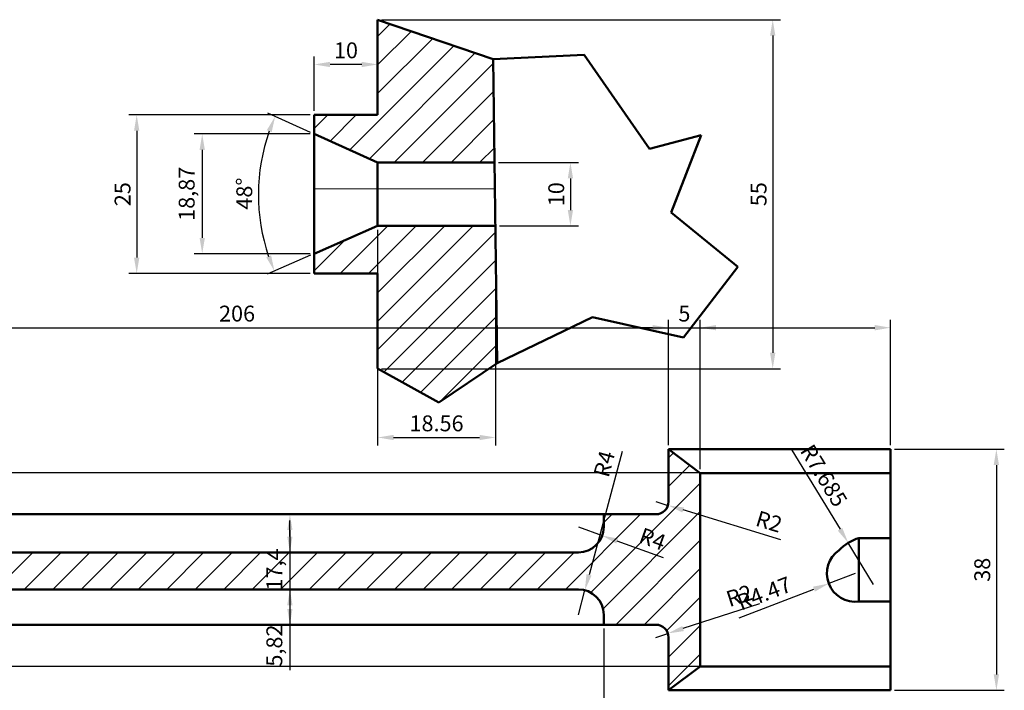
# Model space of a CAD drawing. Units: millimetres. Extents: x 1594 to 1992, y 1694 to 1927.
# Tile 3 of 4: x 1698 to 1853, y 1822 to 1927. Entities that reach past the tile are written whole.
import ezdxf

# ---------------------------------------------------------------- set-up
doc = ezdxf.new("R2010")
doc.units = ezdxf.units.MM
doc.linetypes.add('CENTER', pattern=[50.8, 31.75, -6.35, 6.35, -6.35])
for name, color, linetype, lineweight in [('M-CNTR', 1, 'CENTER', 18), ('M-DIMS', 2, 'Continuous', 25), ('M-HATC', 8, 'Continuous', 18), ('M-OUTL', 7, 'Continuous', 50)]:
    doc.layers.add(name, color=color, linetype=linetype, lineweight=lineweight)
doc.styles.get("Standard").update_dxf_attribs({"font": 'arial.ttf'})
doc.dimstyles.new('ISO-25', dxfattribs={"dimtxt": 2.5, "dimasz": 2.5, "dimexe": 1.25, "dimexo": 0.625, "dimtad": 1, "dimtxsty": 'Standard', "dimcen": 2.5, "dimadec": 0, "dimazin": 0, "dimtfac": 1, "dimtmove": 0, "dimatfit": 3, "dimfxl": 1, "dimarcsym": 0})

# ---------------------------------------------------------------- blocks, each defined once
blk = doc.blocks.new('*D2')
at = {"layer": 'Defpoints', "color": 0, "transparency": 16777216}
for p in [(1834.84, 1859.58), (1834.84, 1821.58), (1851.51, 1821.58)]:
    blk.add_point(p, dxfattribs=at)
at = {"layer": 'M-DIMS', "color": 0, "lineweight": -2, "transparency": 16777216}
for p, q in [((1835.46, 1859.58), (1852.76, 1859.58)), ((1851.51, 1857.08), (1851.51, 1824.08)), ((1835.46, 1821.58), (1852.76, 1821.58))]:
    blk.add_line(p, q, dxfattribs=at)
at = {"layer": 'M-DIMS', "color": 0, "transparency": 16777216}
for points in [[(1851.09, 1857.08), (1851.93, 1857.08), (1851.51, 1859.58)], [(1851.09, 1824.08), (1851.93, 1824.08), (1851.51, 1821.58)]]:
    blk.add_solid(points, dxfattribs=at)
at = {"layer": 'M-DIMS', "color": 0, "transparency": 16777216, "insert": (1849.61, 1840.58), "char_height": 2.5, "attachment_point": 5, "rotation": 90}
blk.add_mtext('38', dxfattribs=at)
blk = doc.blocks.new('*D3')
at = {"layer": 'Defpoints', "color": 0, "transparency": 16777216}
for p in [(1797.84, 1851.32), (1799.75, 1850.73)]:
    blk.add_point(p, dxfattribs=at)
at = {"layer": 'M-DIMS', "color": 0, "lineweight": -2, "transparency": 16777216}
for p, q in [((1797.84, 1851.32), (1799.75, 1850.73)), ((1817.55, 1845.3), (1802.14, 1850))]:
    blk.add_line(p, q, dxfattribs=at)
at = {"layer": 'M-DIMS', "color": 0, "transparency": 16777216}
blk.add_solid([(1802.26, 1850.4), (1802.02, 1849.61), (1799.75, 1850.73)], dxfattribs=at)
at = {"layer": 'M-DIMS', "color": 0, "transparency": 16777216, "insert": (1815.59, 1847.86), "char_height": 2.5, "attachment_point": 5, "rotation": 343.0097}
blk.add_mtext('R2', dxfattribs=at)
blk = doc.blocks.new('*D5')
at = {"layer": 'Defpoints', "color": 0, "transparency": 16777216}
for p in [(1739.34, 1849.32), (1739.34, 1831.92), (1740.17, 1831.92)]:
    blk.add_point(p, dxfattribs=at)
at = {"layer": 'M-DIMS', "color": 0, "lineweight": -2, "transparency": 16777216}
for p, q in [((1739.96, 1849.32), (1741.42, 1849.32)), ((1740.17, 1846.82), (1740.17, 1834.42)), ((1739.96, 1831.92), (1741.42, 1831.92))]:
    blk.add_line(p, q, dxfattribs=at)
at = {"layer": 'M-DIMS', "color": 0, "transparency": 16777216}
for points in [[(1739.75, 1846.82), (1740.58, 1846.82), (1740.17, 1849.32)], [(1739.75, 1834.42), (1740.58, 1834.42), (1740.17, 1831.92)]]:
    blk.add_solid(points, dxfattribs=at)
at = {"layer": 'M-DIMS', "color": 0, "transparency": 16777216, "insert": (1738.04, 1840.62), "char_height": 2.5, "attachment_point": 5, "rotation": 90}
blk.add_mtext('17,4', dxfattribs=at)
blk = doc.blocks.new('*D6')
at = {"layer": 'Defpoints', "color": 0, "transparency": 16777216}
for p in [(1740.17, 1843.32), (1740.17, 1837.49), (1740.17, 1837.49)]:
    blk.add_point(p, dxfattribs=at)
at = {"layer": 'M-DIMS', "color": 0, "lineweight": -2, "transparency": 16777216}
for p, q in [((1740.17, 1845.82), (1740.17, 1848.32)), ((1740.17, 1843.32), (1740.17, 1837.49)), ((1740.79, 1843.32), (1741.42, 1843.32)), ((1740.79, 1837.49), (1741.42, 1837.49)), ((1740.17, 1834.99), (1740.17, 1824.78))]:
    blk.add_line(p, q, dxfattribs=at)
at = {"layer": 'M-DIMS', "color": 0, "transparency": 16777216}
for points in [[(1739.75, 1845.82), (1740.58, 1845.82), (1740.17, 1843.32)], [(1739.75, 1834.99), (1740.58, 1834.99), (1740.17, 1837.49)]]:
    blk.add_solid(points, dxfattribs=at)
at = {"layer": 'M-DIMS', "color": 0, "transparency": 16777216, "insert": (1738.04, 1828.63), "char_height": 2.5, "attachment_point": 5, "rotation": 90}
blk.add_mtext('5,82', dxfattribs=at)
blk = doc.blocks.new('*D7')
at = {"layer": 'Defpoints', "color": 0, "transparency": 16777216}
for p in [(1786.66, 1837.36), (1785.63, 1833.49)]:
    blk.add_point(p, dxfattribs=at)
at = {"layer": 'M-DIMS', "color": 0, "lineweight": -2, "transparency": 16777216}
for p, q in [((1792.51, 1859.24), (1787.31, 1839.77)), ((1785.63, 1833.49), (1786.66, 1837.36))]:
    blk.add_line(p, q, dxfattribs=at)
at = {"layer": 'M-DIMS', "color": 0, "transparency": 16777216}
blk.add_solid([(1786.91, 1839.88), (1787.71, 1839.67), (1786.66, 1837.36)], dxfattribs=at)
at = {"layer": 'M-DIMS', "color": 0, "transparency": 16777216, "insert": (1790.02, 1857.18), "char_height": 2.5, "attachment_point": 5, "rotation": 75.0359}
blk.add_mtext('R4', dxfattribs=at)
blk = doc.blocks.new('*D8')
at = {"layer": 'Defpoints', "color": 0, "transparency": 16777216}
for p in [(1785.63, 1847.32), (1789.39, 1845.96)]:
    blk.add_point(p, dxfattribs=at)
at = {"layer": 'M-DIMS', "color": 0, "lineweight": -2, "transparency": 16777216}
for p, q in [((1785.63, 1847.32), (1789.39, 1845.96)), ((1799.05, 1842.46), (1791.74, 1845.1))]:
    blk.add_line(p, q, dxfattribs=at)
at = {"layer": 'M-DIMS', "color": 0, "transparency": 16777216}
blk.add_solid([(1791.88, 1845.5), (1791.6, 1844.71), (1789.39, 1845.96)], dxfattribs=at)
at = {"layer": 'M-DIMS', "color": 0, "transparency": 16777216, "insert": (1797.21, 1845.12), "char_height": 2.5, "attachment_point": 5, "rotation": 340.0753}
blk.add_mtext('R4', dxfattribs=at)
blk = doc.blocks.new('*D12')
at = {"layer": 'Defpoints', "color": 0, "transparency": 16777216}
for p in [(1797.84, 1829.92), (1799.74, 1830.54)]:
    blk.add_point(p, dxfattribs=at)
at = {"layer": 'M-DIMS', "color": 0, "lineweight": -2, "transparency": 16777216}
for p, q in [((1814.17, 1835.22), (1802.12, 1831.31)), ((1797.84, 1829.92), (1799.74, 1830.54))]:
    blk.add_line(p, q, dxfattribs=at)
at = {"layer": 'M-DIMS', "color": 0, "transparency": 16777216}
blk.add_solid([(1801.99, 1831.71), (1802.25, 1830.91), (1799.74, 1830.54)], dxfattribs=at)
at = {"layer": 'M-DIMS', "color": 0, "transparency": 16777216, "insert": (1811.09, 1836.19), "char_height": 2.5, "attachment_point": 5, "rotation": 17.9685}
blk.add_mtext('R2', dxfattribs=at)
blk = doc.blocks.new('*D34')
at = {"layer": 'Defpoints', "color": 0, "transparency": 16777216}
for p in [(1744, 1909.26), (1754, 1904.77), (1735.52, 1904.02), (1754, 1894.77), (1744, 1890.39)]:
    blk.add_point(p, dxfattribs=at)
at = {"layer": 'M-DIMS', "color": 0, "lineweight": -2, "transparency": 16777216}
for p, q in [((1743.43, 1909.52), (1736.7, 1912.54)), ((1743.43, 1890.14), (1736.59, 1887.15))]:
    blk.add_line(p, q, dxfattribs=at)
blk.add_arc((1765.27, 1899.71), 30.07, 160.5813, 198.8909, dxfattribs=at)
at = {"layer": 'M-DIMS', "color": 0, "transparency": 16777216}
for points in [[(1736.53, 1909.86), (1737.3, 1909.55), (1737.84, 1912.03)], [(1737.21, 1890.13), (1736.44, 1889.83), (1737.73, 1887.65)]]:
    blk.add_solid(points, dxfattribs=at)
at = {"layer": 'M-DIMS', "color": 0, "transparency": 16777216, "insert": (1733.3, 1899.86), "char_height": 2.5, "attachment_point": 5, "rotation": 89.7361}
blk.add_mtext('48°', dxfattribs=at)
blk = doc.blocks.new('*D35')
at = {"layer": 'Defpoints', "color": 0, "transparency": 16777216}
for p in [(1772.42, 1904.77), (1772.56, 1894.77), (1784.38, 1894.77)]:
    blk.add_point(p, dxfattribs=at)
at = {"layer": 'M-DIMS', "color": 0, "lineweight": -2, "transparency": 16777216}
for p, q in [((1773.05, 1904.77), (1785.63, 1904.77)), ((1784.38, 1902.27), (1784.38, 1897.27)), ((1773.18, 1894.77), (1785.63, 1894.77))]:
    blk.add_line(p, q, dxfattribs=at)
at = {"layer": 'M-DIMS', "color": 0, "transparency": 16777216}
for points in [[(1783.96, 1902.27), (1784.79, 1902.27), (1784.38, 1904.77)], [(1783.96, 1897.27), (1784.79, 1897.27), (1784.38, 1894.77)]]:
    blk.add_solid(points, dxfattribs=at)
at = {"layer": 'M-DIMS', "color": 0, "transparency": 16777216, "insert": (1782.47, 1899.77), "char_height": 2.5, "attachment_point": 5, "rotation": 90}
blk.add_mtext('10', dxfattribs=at)
blk = doc.blocks.new('*D36')
at = {"layer": 'Defpoints', "color": 0, "transparency": 16777216}
for p in [(1744, 1909.26), (1726.35, 1890.39), (1744, 1890.39)]:
    blk.add_point(p, dxfattribs=at)
at = {"layer": 'M-DIMS', "color": 0, "lineweight": -2, "transparency": 16777216}
for p, q in [((1743.37, 1909.26), (1725.1, 1909.26)), ((1726.35, 1906.76), (1726.35, 1892.89)), ((1743.37, 1890.39), (1725.1, 1890.39))]:
    blk.add_line(p, q, dxfattribs=at)
at = {"layer": 'M-DIMS', "color": 0, "transparency": 16777216}
for points in [[(1725.93, 1906.76), (1726.77, 1906.76), (1726.35, 1909.26)], [(1725.93, 1892.89), (1726.77, 1892.89), (1726.35, 1890.39)]]:
    blk.add_solid(points, dxfattribs=at)
at = {"layer": 'M-DIMS', "color": 0, "transparency": 16777216, "insert": (1724.22, 1899.83), "char_height": 2.5, "attachment_point": 5, "rotation": 90}
blk.add_mtext('18,87', dxfattribs=at)
blk = doc.blocks.new('*D37')
at = {"layer": 'Defpoints', "color": 0, "transparency": 16777216}
for p in [(1744, 1920.22), (1744, 1912.27), (1754, 1912.27)]:
    blk.add_point(p, dxfattribs=at)
at = {"layer": 'M-DIMS', "color": 0, "lineweight": -2, "transparency": 16777216}
for p, q in [((1744, 1912.9), (1744, 1921.47)), ((1754, 1912.9), (1754, 1921.47)), ((1751.5, 1920.22), (1746.5, 1920.22))]:
    blk.add_line(p, q, dxfattribs=at)
at = {"layer": 'M-DIMS', "color": 0, "transparency": 16777216}
for points in [[(1746.5, 1920.63), (1746.5, 1919.8), (1744, 1920.22)], [(1751.5, 1920.63), (1751.5, 1919.8), (1754, 1920.22)]]:
    blk.add_solid(points, dxfattribs=at)
at = {"layer": 'M-DIMS', "color": 0, "transparency": 16777216, "insert": (1749, 1922.12), "char_height": 2.5, "attachment_point": 5}
blk.add_mtext('10', dxfattribs=at)
blk = doc.blocks.new('*D38')
at = {"layer": 'Defpoints', "color": 0, "transparency": 16777216}
for p in [(1744, 1912.27), (1716.02, 1887.27), (1744, 1887.27)]:
    blk.add_point(p, dxfattribs=at)
at = {"layer": 'M-DIMS', "color": 0, "lineweight": -2, "transparency": 16777216}
for p, q in [((1743.37, 1912.27), (1714.77, 1912.27)), ((1716.02, 1909.77), (1716.02, 1889.77)), ((1743.37, 1887.27), (1714.77, 1887.27))]:
    blk.add_line(p, q, dxfattribs=at)
at = {"layer": 'M-DIMS', "color": 0, "transparency": 16777216}
for points in [[(1715.6, 1909.77), (1716.44, 1909.77), (1716.02, 1912.27)], [(1715.6, 1889.77), (1716.44, 1889.77), (1716.02, 1887.27)]]:
    blk.add_solid(points, dxfattribs=at)
at = {"layer": 'M-DIMS', "color": 0, "transparency": 16777216, "insert": (1714.12, 1899.77), "char_height": 2.5, "attachment_point": 5, "rotation": 90}
blk.add_mtext('25', dxfattribs=at)
blk = doc.blocks.new('*D47')
at = {"layer": 'Defpoints', "color": 0, "transparency": 16777216}
for p in [(1834.84, 1878.73), (1628.84, 1859.58), (1834.84, 1859.58)]:
    blk.add_point(p, dxfattribs=at)
at = {"layer": 'M-DIMS', "color": 0, "lineweight": -2, "transparency": 16777216}
for p, q in [((1628.84, 1860.2), (1628.84, 1879.98)), ((1834.84, 1860.2), (1834.84, 1879.98)), ((1631.34, 1878.73), (1832.34, 1878.73))]:
    blk.add_line(p, q, dxfattribs=at)
at = {"layer": 'M-DIMS', "color": 0, "transparency": 16777216}
for points in [[(1631.34, 1879.15), (1631.34, 1878.31), (1628.84, 1878.73)], [(1832.34, 1879.15), (1832.34, 1878.31), (1834.84, 1878.73)]]:
    blk.add_solid(points, dxfattribs=at)
at = {"layer": 'M-DIMS', "color": 0, "transparency": 16777216, "insert": (1731.84, 1880.63), "char_height": 2.5, "attachment_point": 5}
blk.add_mtext('206', dxfattribs=at)
blk = doc.blocks.new('*D50')
at = {"layer": 'Defpoints', "color": 0, "transparency": 16777216}
for p in [(1690.7, 1831.92), (1789.63, 1831.92), (1789.63, 1695.35)]:
    blk.add_point(p, dxfattribs=at)
at = {"layer": 'M-DIMS', "color": 0, "lineweight": -2, "transparency": 16777216}
for p, q in [((1690.7, 1831.3), (1690.7, 1694.1)), ((1789.63, 1831.3), (1789.63, 1694.1)), ((1693.2, 1695.35), (1787.13, 1695.35))]:
    blk.add_line(p, q, dxfattribs=at)
at = {"layer": 'M-DIMS', "color": 0, "transparency": 16777216}
for points in [[(1693.2, 1695.77), (1693.2, 1694.94), (1690.7, 1695.35)], [(1787.13, 1695.77), (1787.13, 1694.94), (1789.63, 1695.35)]]:
    blk.add_solid(points, dxfattribs=at)
at = {"layer": 'M-DIMS', "color": 0, "transparency": 16777216, "insert": (1740.17, 1697.26), "char_height": 2.5, "attachment_point": 5}
blk.add_mtext('98.93', dxfattribs=at)
blk = doc.blocks.new('*D52')
at = {"layer": 'Defpoints', "color": 0, "transparency": 16777216}
for p in [(1834.84, 1855.83), (1597.57, 1825.34), (1834.84, 1825.34)]:
    blk.add_point(p, dxfattribs=at)
at = {"layer": 'M-DIMS', "color": 0, "lineweight": -2, "transparency": 16777216}
for p, q in [((1834.21, 1855.83), (1596.32, 1855.83)), ((1597.57, 1853.33), (1597.57, 1827.84)), ((1834.21, 1825.34), (1596.32, 1825.34))]:
    blk.add_line(p, q, dxfattribs=at)
at = {"layer": 'M-DIMS', "color": 0, "transparency": 16777216}
for points in [[(1597.15, 1853.33), (1597.99, 1853.33), (1597.57, 1855.83)], [(1597.15, 1827.84), (1597.99, 1827.84), (1597.57, 1825.34)]]:
    blk.add_solid(points, dxfattribs=at)
at = {"layer": 'M-DIMS', "color": 0, "transparency": 16777216, "insert": (1595.67, 1840.58), "char_height": 2.5, "attachment_point": 5, "rotation": 90}
blk.add_mtext('30.49', dxfattribs=at)
blk = doc.blocks.new('*D53')
at = {"layer": 'Defpoints', "color": 0, "transparency": 16777216}
for p in [(1804.84, 1878.73), (1799.84, 1859.58), (1804.84, 1855.83)]:
    blk.add_point(p, dxfattribs=at)
at = {"layer": 'M-DIMS', "color": 0, "lineweight": -2, "transparency": 16777216}
for p, q in [((1799.84, 1860.2), (1799.84, 1879.98)), ((1804.84, 1856.45), (1804.84, 1879.98)), ((1797.34, 1878.73), (1794.84, 1878.73)), ((1799.84, 1878.73), (1804.84, 1878.73)), ((1807.34, 1878.73), (1809.84, 1878.73))]:
    blk.add_line(p, q, dxfattribs=at)
at = {"layer": 'M-DIMS', "color": 0, "transparency": 16777216}
for points in [[(1797.34, 1879.15), (1797.34, 1878.31), (1799.84, 1878.73)], [(1807.34, 1879.15), (1807.34, 1878.31), (1804.84, 1878.73)]]:
    blk.add_solid(points, dxfattribs=at)
at = {"layer": 'M-DIMS', "color": 0, "transparency": 16777216, "insert": (1802.34, 1880.63), "char_height": 2.5, "attachment_point": 5}
blk.add_mtext('5', dxfattribs=at)
blk = doc.blocks.new('*D56')
at = {"layer": 'Defpoints', "color": 0, "transparency": 16777216}
for p in [(1754, 1894.77), (1772.56, 1894.77), (1772.56, 1861.43)]:
    blk.add_point(p, dxfattribs=at)
at = {"layer": 'M-DIMS', "color": 0, "lineweight": -2, "transparency": 16777216}
for p, q in [((1754, 1894.15), (1754, 1860.18)), ((1772.56, 1894.15), (1772.56, 1860.18)), ((1756.5, 1861.43), (1770.06, 1861.43))]:
    blk.add_line(p, q, dxfattribs=at)
at = {"layer": 'M-DIMS', "color": 0, "transparency": 16777216}
for points in [[(1756.5, 1861.84), (1756.5, 1861.01), (1754, 1861.43)], [(1770.06, 1861.84), (1770.06, 1861.01), (1772.56, 1861.43)]]:
    blk.add_solid(points, dxfattribs=at)
at = {"layer": 'M-DIMS', "color": 0, "transparency": 16777216, "insert": (1763.28, 1863.33), "char_height": 2.5, "attachment_point": 5}
blk.add_mtext('18.56', dxfattribs=at)
blk = doc.blocks.new('*D57')
at = {"layer": 'Defpoints', "color": 0, "transparency": 16777216}
for p in [(1754, 1927.27), (1754, 1872.27), (1816.26, 1872.27)]:
    blk.add_point(p, dxfattribs=at)
at = {"layer": 'M-DIMS', "color": 0, "lineweight": -2, "transparency": 16777216}
for p, q in [((1754.62, 1927.27), (1817.51, 1927.27)), ((1816.26, 1924.77), (1816.26, 1874.77)), ((1754.62, 1872.27), (1817.51, 1872.27))]:
    blk.add_line(p, q, dxfattribs=at)
at = {"layer": 'M-DIMS', "color": 0, "transparency": 16777216}
for points in [[(1815.84, 1924.77), (1816.68, 1924.77), (1816.26, 1927.27)], [(1815.84, 1874.77), (1816.68, 1874.77), (1816.26, 1872.27)]]:
    blk.add_solid(points, dxfattribs=at)
at = {"layer": 'M-DIMS', "color": 0, "transparency": 16777216, "insert": (1814.36, 1899.77), "char_height": 2.5, "attachment_point": 5, "rotation": 90}
blk.add_mtext('55', dxfattribs=at)
blk = doc.blocks.new('*D65')
at = {"layer": 'Defpoints', "color": 0, "transparency": 16777216}
for p in [(1828.17, 1844.82), (1832.16, 1838.25)]:
    blk.add_point(p, dxfattribs=at)
at = {"layer": 'M-DIMS', "color": 0, "lineweight": -2, "transparency": 16777216}
for p, q in [((1819.29, 1859.43), (1826.87, 1846.96)), ((1832.16, 1838.25), (1828.17, 1844.82))]:
    blk.add_line(p, q, dxfattribs=at)
at = {"layer": 'M-DIMS', "color": 0, "transparency": 16777216}
blk.add_solid([(1827.23, 1847.17), (1826.52, 1846.74), (1828.17, 1844.82)], dxfattribs=at)
at = {"layer": 'M-DIMS', "color": 0, "transparency": 16777216, "insert": (1824.05, 1855.25), "char_height": 2.5, "attachment_point": 5, "rotation": 301.3058}
blk.add_mtext('R7.685', dxfattribs=at)
blk = doc.blocks.new('*D66')
at = {"layer": 'Defpoints', "color": 0, "transparency": 16777216}
for p in [(1829.27, 1840.01), (1825.1, 1838.41)]:
    blk.add_point(p, dxfattribs=at)
at = {"layer": 'M-DIMS', "color": 0, "lineweight": -2, "transparency": 16777216}
for p, q in [((1829.27, 1840.01), (1825.1, 1838.41)), ((1810.97, 1832.99), (1822.76, 1837.52))]:
    blk.add_line(p, q, dxfattribs=at)
at = {"layer": 'M-DIMS', "color": 0, "transparency": 16777216}
blk.add_solid([(1822.62, 1837.91), (1822.91, 1837.13), (1825.1, 1838.41)], dxfattribs=at)
at = {"layer": 'M-DIMS', "color": 0, "transparency": 16777216, "insert": (1815.03, 1836.56), "char_height": 2.5, "attachment_point": 5, "rotation": 20.9765}
blk.add_mtext('R4.47', dxfattribs=at)

msp = doc.modelspace()

# ---------------------------------------------------------------- hatches: boundary and pattern name
at = {"layer": 'M-HATC'}
h = msp.add_hatch(dxfattribs=at)
h.set_pattern_fill('ANSI31', color=256)
h.paths.add_polyline_path([(1772.2059, 1921.0678), (1753.9999, 1927.2738), (1753.9999, 1912.2738), (1743.9999, 1912.2738), (1743.9999, 1909.2647), (1753.9999, 1904.7738), (1772.4244, 1904.7738)])
h.paths.add_polyline_path([(1772.5584, 1894.7738), (1753.9999, 1894.7738), (1743.9999, 1890.3932), (1743.9999, 1887.2738), (1753.9999, 1887.2738), (1753.9999, 1872.2738), (1763.6384, 1866.9253), (1772.8485, 1873.1313)])
h = msp.add_hatch(dxfattribs=at)
h.set_pattern_fill('ANSI31', color=256)
h.paths.add_polyline_path([(1804.8392, 1855.8272), (1799.8392, 1859.5797), (1799.8392, 1854.5797), (1799.8392, 1851.3192, -0.41421356), (1797.8392, 1849.3192), (1789.6319, 1849.3192), (1789.6319, 1847.3189, -0.41421356), (1785.6319, 1843.3189), (1694.7029, 1843.3189, -0.41421356), (1690.7029, 1847.3189), (1690.7029, 1849.3192), (1680.8392, 1849.3192, -0.41421356), (1678.8392, 1851.3192), (1678.8392, 1859.5797), (1673.8392, 1859.5797), (1673.8392, 1821.5797), (1678.8392, 1821.5797), (1678.8392, 1829.9212, -0.41421356), (1680.8392, 1831.9212), (1690.7029, 1831.9212), (1690.7029, 1833.4941, -0.41421356), (1694.7029, 1837.4941), (1785.6319, 1837.4941, -0.41421356), (1789.6319, 1833.4941), (1789.6319, 1831.9212), (1797.8392, 1831.9212, -0.41421356), (1799.8392, 1829.9212), (1799.8392, 1826.5797), (1799.8392, 1821.5797), (1804.8392, 1825.339)])

# ---------------------------------------------------------------- linework, layer by layer
at = {"layer": 'M-CNTR'}
msp.add_line((1772.4803, 1900.5982), (1743.9999, 1900.5982), dxfattribs=at)
at = {"layer": 'M-OUTL'}
for p, q in [((1753.9999, 1927.2738), (1753.9999, 1912.2738)), ((1753.9999, 1927.2738), (1772.2059, 1921.0678)), ((1772.2059, 1921.0678), (1786.5566, 1921.7098)), ((1786.5566, 1921.7098), (1796.8377, 1906.9436)), ((1772.2059, 1921.0678), (1772.8485, 1873.1313)), ((1753.9999, 1912.2738), (1743.9999, 1912.2738)), ((1743.9999, 1912.2738), (1743.9999, 1887.2738)), ((1753.9999, 1904.7738), (1743.9999, 1909.2647)), ((1796.8377, 1906.9436), (1804.9768, 1909.0837)), ((1804.9768, 1909.0837), (1800.2647, 1896.8856)), ((1753.9999, 1904.7738), (1772.4244, 1904.7738)), ((1753.9999, 1904.7738), (1753.9999, 1894.7738)), ((1772.5272, 1900.5996), (1772.4803, 1900.5982)), ((1800.2647, 1896.8856), (1810.76, 1888.3255)), ((1753.9999, 1894.7738), (1743.9999, 1890.3932)), ((1772.5584, 1894.7738), (1753.9999, 1894.7738)), ((1737.8505, 1887.6994), (1737.8505, 1887.6994)), ((1743.9999, 1887.2738), (1753.9999, 1887.2738)), ((1753.9999, 1887.2738), (1753.9999, 1872.2738)), ((1810.76, 1888.3255), (1802.1924, 1877.1974)), ((1787.8417, 1880.4074), (1772.8485, 1873.1313)), ((1802.1924, 1877.1974), (1787.8417, 1880.4074)), ((1763.6384, 1866.9253), (1772.8485, 1873.1313)), ((1753.9999, 1872.2738), (1763.6384, 1866.9253)), ((1799.8392, 1854.5797), (1799.8392, 1859.5797)), ((1799.8392, 1859.5797), (1834.8392, 1859.5797)), ((1799.8392, 1859.5797), (1804.8392, 1859.5797)), ((1804.8392, 1855.8272), (1799.8392, 1859.5797)), ((1834.8392, 1859.5797), (1834.8392, 1821.5797)), ((1799.8392, 1851.3192), (1799.8392, 1854.5797)), ((1804.8392, 1855.8272), (1804.8392, 1825.339)), ((1804.8392, 1855.8272), (1834.8392, 1855.8272)), ((1680.8392, 1849.3192), (1797.8392, 1849.3192)), ((1789.6319, 1847.3189), (1789.6319, 1849.3192)), ((1834.8392, 1845.5797), (1829.8392, 1845.5797)), ((1829.8392, 1835.5797), (1829.8392, 1845.5797)), ((1834.8392, 1840.5797), (1834.8392, 1845.5797)), ((1834.8392, 1845.5797), (1834.8392, 1835.5797)), ((1694.7029, 1843.3189), (1785.6319, 1843.3189)), ((1694.7029, 1837.4941), (1785.6319, 1837.4941)), ((1834.8392, 1835.5797), (1829.8392, 1835.5797)), ((1789.6319, 1833.4941), (1789.6319, 1831.9212)), ((1797.8392, 1831.9212), (1680.8392, 1831.9212)), ((1799.8392, 1826.5797), (1799.8392, 1829.9212)), ((1799.8392, 1821.5797), (1799.8392, 1826.5797)), ((1804.8392, 1825.339), (1799.8392, 1821.5797)), ((1834.8392, 1825.339), (1804.8392, 1825.339)), ((1834.8392, 1821.5797), (1799.8392, 1821.5797))]:
    msp.add_line(p, q, dxfattribs=at)
for centre, radius, start, end in [((1797.8392, 1851.3192), 2, 270, 0), ((1785.6319, 1847.3189), 4, 270, 0), ((1832.1644, 1838.2544), 7.6855, 107.611167, 135), ((1829.2726, 1840.0131), 4.4695, 124.671968, 277.283134), ((1785.6319, 1833.4941), 4, 0, 90), ((1797.8392, 1829.9212), 2, 0, 90)]:
    msp.add_arc(centre, radius, start, end, dxfattribs=at)

# ---------------------------------------------------------------- dimensions: what is measured, and where the dimension line sits
at = {"layer": 'M-DIMS'}
for base, p1, p2, override, picture, middle in [((1816.26, 1872.2738), (1753.9999, 1927.2738), (1753.9999, 1872.2738), {"dimdec": 0, "dimlfac": 1, "dimrnd": 0, "dimzin": 0, "dimdsep": 46, "dimlunit": 2}, '*D57', (1814.3636, 1899.7738)), ((1716.019, 1887.2738), (1743.9999, 1912.2738), (1743.9999, 1887.2738), {"dimclrd": 0, "dimclre": 0, "dimclrt": 0}, '*D38', (1714.1175, 1899.7738)), ((1726.3486, 1890.3932), (1743.9999, 1909.2647), (1743.9999, 1890.3932), {"dimclrd": 0, "dimclre": 0, "dimclrt": 0}, '*D36', (1724.2213, 1899.8289)), ((1784.3754, 1894.7738), (1772.4244, 1904.7738), (1772.5584, 1894.7738), {"dimclrd": 0, "dimclre": 0, "dimclrt": 0}, '*D35', (1782.474, 1899.7738)), ((1851.5106, 1821.5797), (1834.8392, 1859.5797), (1834.8392, 1821.5797), {"dimclrd": 0, "dimclre": 0, "dimclrt": 0}, '*D2', (1849.6084, 1840.5797)), ((1597.571, 1825.339), (1834.8392, 1855.8272), (1834.8392, 1825.339), {"dimdec": 2, "dimlfac": 1, "dimrnd": 0, "dimzin": 0, "dimdsep": 46, "dimlunit": 2}, '*D52', (1595.6687, 1840.5831)), ((1740.1674, 1831.9212), (1739.3392, 1849.3192), (1739.3392, 1831.9212), {"dimclrd": 0, "dimclre": 0, "dimclrt": 0}, '*D5', (1738.04, 1840.6202)), ((1740.1674, 1837.4941), (1740.1674, 1843.3189), (1740.1674, 1837.4941), {"dimclrd": 0, "dimclre": 0, "dimclrt": 0}, '*D6', (1738.04, 1828.635))]:
    dim = msp.add_linear_dim(base=base, p1=p1, p2=p2, angle=90, dimstyle='ISO-25', override=override, dxfattribs=at)
    dim.commit()
    dim.dimension.update_dxf_attribs({"geometry": picture, "text_midpoint": middle})
for base, p1, p2, override, picture, middle in [((1743.9999, 1920.2151), (1753.9999, 1912.2738), (1743.9999, 1912.2738), {"dimclrd": 0, "dimclre": 0, "dimclrt": 0}, '*D37', (1748.9999, 1922.1165)), ((1772.5584, 1861.4253), (1753.9999, 1894.7738), (1772.5584, 1894.7738), {"dimdec": 2, "dimlfac": 1, "dimrnd": 0, "dimzin": 0, "dimdsep": 46, "dimlunit": 2}, '*D56', (1763.2791, 1863.3267)), ((1834.8392, 1878.7297), (1628.8392, 1859.5797), (1834.8392, 1859.5797), {"dimdec": 0, "dimlfac": 1, "dimrnd": 0, "dimzin": 0, "dimdsep": 46, "dimlunit": 2}, '*D47', (1731.8392, 1880.6312)), ((1804.8392, 1878.7297), (1799.8392, 1859.5797), (1804.8392, 1855.8272), {"dimdec": 0, "dimlfac": 1, "dimrnd": 0, "dimzin": 0, "dimdsep": 46, "dimlunit": 2}, '*D53', (1802.3392, 1880.626)), ((1789.6319, 1695.3548), (1690.7029, 1831.9212), (1789.6319, 1831.9212), {"dimdec": 2, "dimlfac": 1, "dimrnd": 0, "dimzin": 0, "dimdsep": 46, "dimlunit": 2}, '*D50', (1740.1674, 1697.2571))]:
    dim = msp.add_linear_dim(base=base, p1=p1, p2=p2, dimstyle='ISO-25', override=override, dxfattribs=at)
    dim.commit()
    dim.dimension.update_dxf_attribs({"geometry": picture, "text_midpoint": middle})
dim = msp.add_angular_dim_2l(base=(1735.5154, 1904.0195), line1=((1753.9999, 1894.7738), (1743.9999, 1890.3932)), line2=((1753.9999, 1904.7738), (1743.9999, 1909.2647)), dimstyle='ISO-25', override={"dimclrd": 0, "dimclre": 0, "dimclrt": 0}, dxfattribs=at)
dim.commit()
dim.dimension.update_dxf_attribs({"geometry": '*D34', "text_midpoint": (1733.3042, 1899.8589)})
for center, mpoint, override, picture, middle in [((1832.164448, 1838.25443), (1828.171021, 1844.820966), {"dimdec": 3, "dimlfac": 1, "dimrnd": 0, "dimzin": 0, "dimdsep": 46, "dimlunit": 2}, '*D65', (1824.054613, 1855.249101)), ((1785.6319, 1847.3189), (1789.3924, 1845.9557), {"dimclrd": 0, "dimclre": 0, "dimclrt": 0}, '*D8', (1797.2099, 1845.1164)), ((1829.2726, 1840.0131), (1825.0993, 1838.4131), {"dimdec": 2, "dimlfac": 1, "dimrnd": 0, "dimzin": 0, "dimdsep": 46, "dimlunit": 2}, '*D66', (1815.0271, 1836.5596))]:
    dim = msp.add_radius_dim(center=center, mpoint=mpoint, dimstyle='ISO-25', override=override, dxfattribs=at)
    dim.commit()
    dim.dimension.update_dxf_attribs({"geometry": picture, "text_midpoint": middle})
for center, mpoint, picture, middle in [((1785.6319, 1833.4941), (1786.6647, 1837.3585), '*D7', (1791.832, 1856.6913)), ((1797.8392, 1851.3192), (1799.7519, 1850.7348), '*D3', (1815.0403, 1846.0635)), ((1797.8392, 1829.9212), (1799.7416, 1830.5382), '*D12', (1811.6688, 1834.4064))]:
    dim = msp.add_radius_dim(center=center, mpoint=mpoint, dimstyle='ISO-25', override={"dimclrd": 0, "dimclre": 0, "dimclrt": 0}, dxfattribs=at)
    dim.commit()
    dim.dimension.update_dxf_attribs({"geometry": picture, "text_midpoint": middle, "dimtype": 164})

doc.saveas('drawing.dxf')
